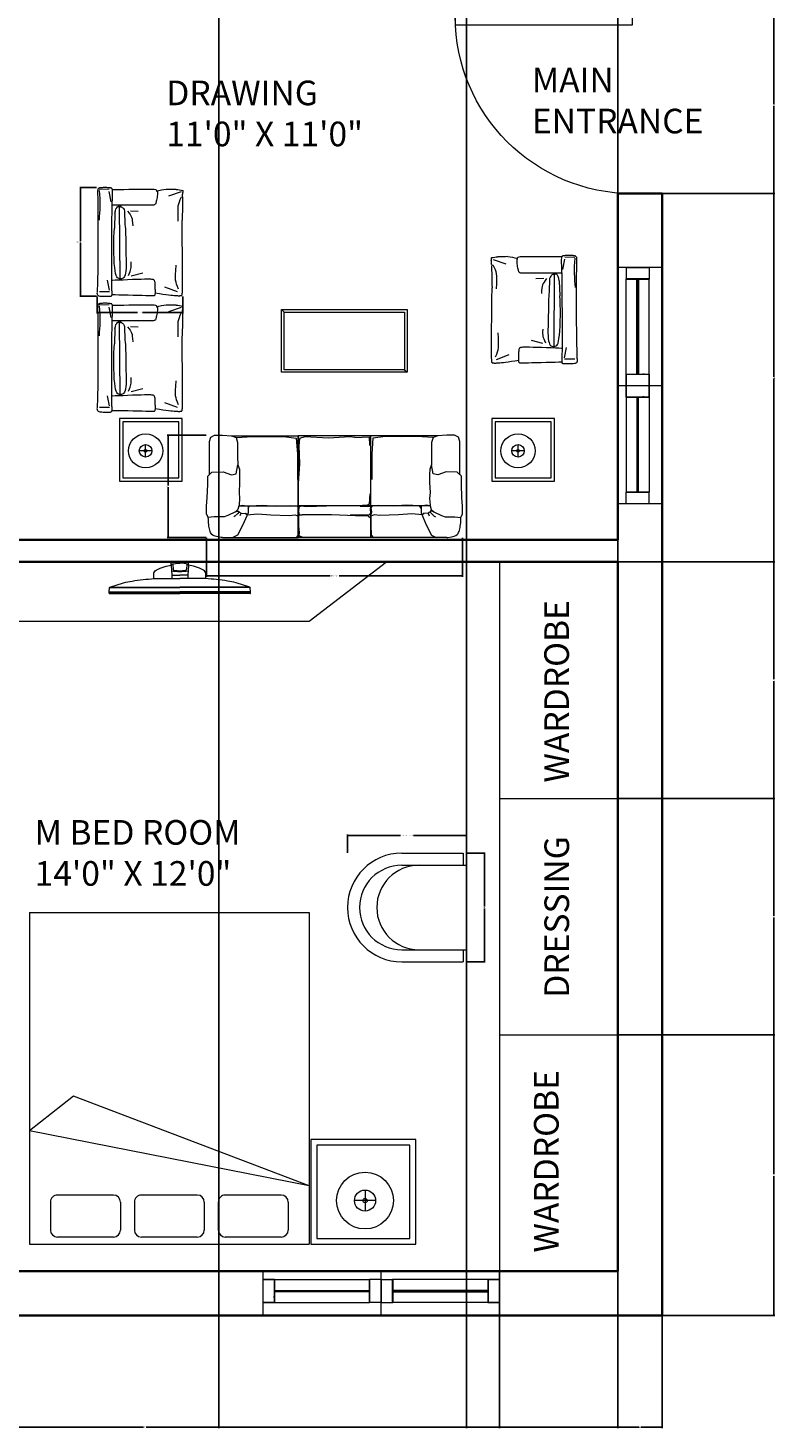
# Model space of a CAD drawing. Units: inches. Extents: x 1723 to 2209, y 1326 to 1810.
# Tile 5 of 6: x 2057 to 2209, y 1326 to 1610. Entities that reach past the tile are written whole.
import ezdxf

# ---------------------------------------------------------------- set-up
doc = ezdxf.new("R2010")
doc.units = ezdxf.units.IN
doc.layers.get('Defpoints').update_dxf_attribs({"color": 255})
for name, color, linetype, lineweight in [('A-ANNO-DIMS', 2, 'Continuous', 18), ('A-ANNO-TEXT', 7, 'Continuous', 18), ('A-AREA-IDEN', 7, 'Continuous', 18), ('A-DOOR', 3, 'Continuous', 18), ('A-EQPM', 8, 'Continuous', 13), ('A-FLOR-CASE', 9, 'Continuous', 18), ('A-FURN', 8, 'Continuous', 13), ('A-GLAZ', 4, 'Continuous', 18), ('A-WALL', 7, 'Continuous', 35), ('Sliding Door', 3, 'Continuous', 18)]:
    doc.layers.add(name, color=color, linetype=linetype, lineweight=lineweight)
doc.styles.get("Standard").update_dxf_attribs({"font": 'arial.ttf'})
doc.dimstyles.get("Standard").update_dxf_attribs({"dimtxt": 0.18, "dimasz": 0.18, "dimexe": 0.18, "dimexo": 0.0625, "dimgap": 0.09, "dimtad": 0, "dimtih": 1, "dimtoh": 1, "dimdec": 4, "dimzin": 0, "dimdsep": 46, "dimtxsty": 'Standard', "dimcen": 0.09, "dimadec": 0, "dimazin": 0, "dimtfac": 1, "dimtdec": 4, "dimtofl": 0, "dimtmove": 0, "dimatfit": 3, "dimfxl": 1, "dimtolj": 1, "dimtzin": 0, "dimarcsym": 0})

# ---------------------------------------------------------------- blocks, each defined once
blk = doc.blocks.new('armchair 042')
at = {"color": 0}
for p, q in [((672, 990), (673, 1002)), ((672, 985), (672, 990)), ((677, 823), (672, 985)), ((673, 1010), (674, 1014)), ((673, 1002), (673, 1010)), ((674, 1014), (675, 1017)), ((675, 1017), (676, 1020)), ((676, 1020), (678, 1023)), ((678, 1023), (680, 1025)), ((680, 1025), (684, 1026)), ((684, 1026), (688, 1027)), ((688, 1027), (694, 1029)), ((694, 1029), (700, 1029)), ((700, 1029), (709, 1030)), ((709, 1030), (718, 1030)), ((718, 1030), (728, 1031)), ((728, 1031), (739, 1031)), ((739, 1031), (750, 1031)), ((750, 1031), (760, 1031)), ((760, 1031), (770, 1030)), ((770, 1030), (779, 1030)), ((779, 1030), (787, 1029)), ((787, 1029), (793, 1028)), ((793, 1028), (798, 1027)), ((798, 1027), (803, 1025)), ((803, 1025), (806, 1023)), ((806, 1023), (809, 1020)), ((809, 1020), (811, 1016)), ((811, 1016), (813, 1011)), ((813, 1011), (814, 1005)), ((815, 997), (813, 908)), ((814, 1005), (815, 997)), ((557, 808), (554, 678)), ((562, 820), (557, 808)), ((568, 830), (562, 820)), ((574, 837), (568, 830)), ((580, 842), (574, 837)), ((587, 846), (580, 842)), ((595, 848), (587, 846)), ((599, 854), (591, 853)), ((602, 850), (595, 848)), ((607, 855), (599, 854)), ((610, 850), (602, 850)), ((614, 854), (607, 855)), ((618, 849), (610, 850)), ((622, 850), (614, 854)), ((625, 846), (618, 849)), ((629, 843), (622, 850)), ((632, 839), (625, 846)), ((639, 827), (632, 839)), ((645, 810), (639, 827)), ((650, 786), (645, 810)), ((678, 701), (677, 823)), ((812, 827), (811, 762)), ((813, 908), (812, 827)), ((7, 656), (8, 675)), ((8, 714), (8, 718)), ((8, 709), (8, 714)), ((8, 690), (8, 709)), ((8, 675), (8, 690)), ((554, 678), (551, 659)), ((650, 786), (654, 642)), ((679, 584), (678, 701)), ((811, 762), (811, 680)), ((811, 680), (811, 600)), ((7, 632), (7, 656)), ((7, 602), (7, 632)), ((7, 567), (7, 602)), ((7, 528), (7, 567)), ((547, 584), (546, 554)), ((546, 554), (546, 523)), ((548, 612), (547, 584)), ((549, 637), (548, 612)), ((551, 659), (549, 637)), ((657, 603), (654, 642)), ((659, 557), (657, 603)), ((660, 507), (659, 557)), ((680, 474), (679, 584)), ((811, 600), (812, 523)), ((4, 359), (5, 404)), ((5, 404), (7, 528)), ((545, 421), (544, 386)), ((546, 490), (545, 456)), ((545, 456), (545, 421)), ((546, 523), (546, 490)), ((657, 353), (659, 403)), ((659, 403), (660, 455)), ((660, 455), (660, 507)), ((680, 378), (680, 474)), ((812, 523), (812, 450)), ((812, 450), (812, 381)), ((4, 316), (4, 359)), ((4, 275), (4, 316)), ((4, 237), (4, 275)), ((543, 352), (542, 319)), ((542, 319), (542, 288)), ((542, 288), (543, 260)), ((544, 386), (543, 352)), ((651, 267), (655, 307)), ((655, 307), (657, 353)), ((680, 298), (680, 378)), ((680, 233), (680, 298)), ((812, 381), (813, 318)), ((813, 318), (813, 261)), ((4, 203), (4, 237)), ((4, 172), (4, 203)), ((4, 145), (4, 172)), ((4, 123), (4, 145)), ((543, 260), (545, 234)), ((545, 234), (548, 213)), ((548, 213), (552, 196)), ((552, 196), (558, 183)), ((558, 183), (564, 173)), ((564, 173), (572, 166)), ((572, 166), (579, 162)), ((579, 162), (588, 160)), ((588, 160), (596, 159)), ((596, 159), (604, 160)), ((604, 160), (611, 161)), ((611, 161), (619, 164)), ((619, 164), (625, 169)), ((625, 169), (632, 178)), ((632, 178), (638, 191)), ((638, 191), (643, 210)), ((643, 210), (647, 235)), ((647, 235), (651, 267)), ((680, 182), (680, 233)), ((680, 143), (680, 182)), ((680, 113), (680, 143)), ((813, 261), (814, 212)), ((814, 212), (815, 171)), ((815, 171), (816, 137)), ((816, 137), (816, 110)), ((4, 105), (4, 123)), ((4, 90), (4, 105)), ((4, 78), (4, 90)), ((4, 69), (4, 78)), ((4, 61), (4, 69)), ((4, 54), (4, 61)), ((4, 48), (4, 54)), ((4, 43), (4, 48)), ((5, 37), (4, 43)), ((5, 31), (5, 37)), ((5, 26), (5, 31)), ((6, 21), (5, 26)), ((6, 16), (6, 21)), ((7, 12), (6, 16)), ((7, 9), (7, 12)), ((8, 6), (7, 9)), ((9, 4), (8, 6)), ((9, 3), (9, 4)), ((10, 2), (9, 3)), ((11, 1), (10, 2)), ((12, 1), (11, 1)), ((13, 1), (12, 1)), ((14, 1), (13, 1)), ((15, 0), (14, 1)), ((16, 0), (15, 0)), ((18, 0), (16, 0)), ((70, 0), (59, -1)), ((82, 1), (70, 0)), ((98, 3), (82, 1)), ((116, 4), (98, 3)), ((137, 7), (116, 4)), ((163, 10), (137, 7)), ((192, 14), (163, 10)), ((225, 19), (192, 14)), ((264, 24), (225, 19)), ((677, 37), (678, 48)), ((677, 28), (677, 37)), ((677, 20), (677, 28)), ((677, 13), (677, 20)), ((677, 8), (677, 13)), ((678, 3), (677, 8)), ((678, 60), (679, 73)), ((678, 48), (678, 60)), ((679, -1), (678, 3)), ((679, 90), (680, 113)), ((679, 73), (679, 90)), ((797, 39), (701, 38)), ((814, 3), (809, 0)), ((817, 7), (814, 3)), ((816, 110), (817, 88)), ((817, 88), (818, 71)), ((819, 12), (817, 7)), ((818, 71), (819, 58)), ((819, 58), (819, 47)), ((819, 47), (820, 39)), ((820, 17), (819, 12)), ((820, 39), (820, 31)), ((820, 31), (821, 24)), ((821, 24), (820, 17)), ((19, 0), (18, 0)), ((21, -1), (19, 0)), ((23, -1), (21, -1)), ((25, -1), (23, -1)), ((27, -1), (25, -1)), ((29, -2), (27, -1)), ((31, -2), (29, -2)), ((35, -2), (31, -2)), ((39, -2), (35, -2)), ((44, -2), (39, -2)), ((51, -1), (44, -2)), ((59, -1), (51, -1)), ((681, -3), (679, -1)), ((684, -5), (681, -3)), ((687, -7), (684, -5)), ((691, -8), (687, -7)), ((696, -8), (691, -8)), ((702, -8), (696, -8)), ((709, -8), (702, -8)), ((718, -8), (709, -8)), ((728, -8), (718, -8)), ((739, -8), (728, -8)), ((750, -8), (739, -8)), ((762, -8), (750, -8)), ((773, -7), (762, -8)), ((784, -6), (773, -7)), ((794, -5), (784, -6)), ((802, -3), (794, -5)), ((809, 0), (802, -3))]:
    blk.add_line(p, q, dxfattribs=at)
for points in [[(16, 939), (28, 914), (37, 893), (43, 874), (47, 854), (49, 830), (50, 800), (49, 761), (47, 710)], [(17, 991), (139, 950)], [(674, 1014), (664, 1014), (641, 1014), (606, 1014), (564, 1014), (517, 1015), (468, 1015), (421, 1016), (378, 1016), (343, 1016), (314, 1016), (292, 1016), (275, 1015), (263, 1012), (254, 1008), (249, 1003), (245, 996), (244, 986), (243, 975), (244, 962), (245, 949), (247, 936), (249, 923), (252, 911), (254, 901), (256, 892), (258, 885), (259, 879), (261, 874), (264, 871), (267, 868), (270, 866), (274, 865), (280, 864), (291, 863), (310, 862), (343, 862), (391, 862), (460, 862), (553, 863), (673, 864)], [(685, 895), (703, 994)], [(703, 1015), (799, 1013)], [(799, 1004), (795, 964), (792, 926), (792, 890), (792, 855), (794, 820), (796, 787), (799, 754), (801, 721)], [(502, 809), (426, 805)], [(529, 807), (514, 788), (504, 773), (496, 760), (490, 747), (486, 733), (484, 715), (481, 693), (479, 664)], [(600, 160), (605, 850)], [(41, 60), (53, 85), (61, 107), (66, 126), (70, 146), (71, 170), (70, 200), (68, 239), (65, 290)], [(520, 191), (511, 212), (504, 229), (499, 243), (496, 256), (495, 268), (494, 283), (494, 301), (495, 323)], [(677, 8), (669, 8), (646, 8), (612, 7), (570, 6), (524, 5), (476, 4), (430, 3), (389, 2), (355, 1), (329, 0), (309, -1), (294, -1), (284, -1), (277, -1), (272, 0), (269, 2), (267, 4), (266, 7), (265, 11), (264, 16), (263, 22), (263, 28), (263, 35), (263, 43), (263, 52), (264, 61), (264, 71), (264, 81), (264, 90), (265, 100), (265, 108), (266, 116), (266, 123), (267, 129), (268, 134), (270, 139), (271, 142), (273, 145), (276, 148), (279, 150), (283, 152), (288, 153), (296, 154), (306, 155), (321, 156), (341, 156), (366, 155), (399, 154), (438, 153), (482, 152), (528, 150), (572, 148), (613, 146), (647, 145), (671, 144), (680, 144)], [(493, 189), (384, 216)], [(701, 50), (720, 148)], [(51, 36), (172, 81)]]:
    blk.add_lwpolyline(points, dxfattribs=at)
for centre, radius, start, end in [((57, 993), 57, 170.3495, 189.4629), ((4, 1002), 3.43, 101.0702, 170.3495), ((-256, 941), 260, 0.5509, 9.4629), ((159, 182), 837, 96.5918, 100.7196), ((4370, 902), 4366, 179.458, 182.4099), ((770, -30414), 31437, 91.1145, 91.2881), ((118, 571), 447, 72.4885, 84.8095)]:
    blk.add_arc(centre, radius, start, end, dxfattribs=at)
blk = doc.blocks.new('sofa 053')
at = {"color": 0}
for p, q in [((-920, 900), (188, 900)), ((-326, 0), (-326, 900)), ((-318, 814), (-313, 892)), ((-185, 886), (-313, 892)), ((-185, 886), (-140, 891)), ((-140, 891), (49, 880)), ((49, 880), (260, 891)), ((188, 900), (317, 900)), ((260, 891), (306, 877)), ((306, 877), (311, 812)), ((317, 0), (317, 900)), ((317, 900), (317, 0)), ((910, 900), (317, 900)), ((311, 812), (306, 652)), ((306, 652), (317, 477)), ((-851, 280), (188, 280)), ((188, 280), (317, 280)), ((842, 280), (317, 280)), ((143, 201), (209, 202)), ((209, 202), (282, 201)), ((-998, 0), (188, 0)), ((188, 0), (317, 0)), ((989, 0), (317, 0))]:
    blk.add_line(p, q, dxfattribs=at)
for points in [[(-1112, 556), (-1113, 849), (-1101, 889), (-1067, 906), (-997, 906), (-918, 900), (-876, 886), (-864, 841), (-864, 717), (-862, 643)], [(-876, 886), (-729, 894)], [(-598, 891), (-455, 894), (-344, 880), (-333, 742), (-333, 513)], [(720, 894), (445, 894), (335, 880), (324, 742), (324, 513)], [(866, 886), (720, 894)], [(1103, 556), (1103, 849), (1092, 889), (1058, 906), (988, 906), (909, 900), (866, 886), (855, 841), (855, 717), (853, 643)], [(-983, 183), (-1070, 183), (-1123, 178), (-1138, 209), (-1138, 277), (-1132, 353), (-1127, 468), (-1127, 542), (-1090, 578), (-991, 581), (-918, 556), (-876, 564), (-862, 643), (-862, 643), (-847, 601)], [(-862, 643), (-847, 606), (-845, 554), (-845, 488), (-850, 397), (-845, 345), (-850, 286), (-851, 280)], [(853, 643), (838, 606), (836, 554), (836, 488), (840, 397), (836, 345), (840, 286), (842, 280)], [(974, 183), (1061, 183), (1114, 178), (1129, 209), (1129, 277), (1123, 353), (1118, 468), (1118, 542), (1081, 578), (982, 581), (909, 556), (866, 564), (853, 643), (853, 643), (838, 601)], [(-318, 388), (-312, 296), (-300, 287), (-202, 280)], [(-851, 280), (-861, 248), (-882, 227), (-951, 195), (-983, 183)], [(-851, 280), (-819, 285), (-771, 277), (-771, 217), (-816, 113), (-864, 20), (-904, 0)], [(-771, 259), (-757, 279), (-639, 285), (-522, 278), (-394, 284), (-337, 281), (-326, 262), (-331, 225), (-326, 200)], [(-142, 202), (-318, 205), (-326, 215), (-322, 250), (-325, 271), (-230, 275)], [(67, 277), (241, 272), (295, 278), (313, 269), (316, 229), (310, 202), (282, 201), (314, 195), (317, 133), (310, 42), (312, 18), (286, 5)], [(762, 259), (748, 279), (630, 285), (513, 278), (385, 284), (327, 281), (317, 262), (321, 225), (317, 200)], [(842, 280), (810, 285), (762, 277), (762, 217), (807, 113), (855, 20), (895, 0)], [(842, 280), (852, 248), (873, 227), (942, 195), (974, 183)], [(-998, 0), (-1008, 1), (-1039, 6), (-1062, 12), (-1079, 19), (-1091, 26), (-1098, 35), (-1103, 44), (-1107, 54), (-1110, 65), (-1113, 76), (-1115, 88), (-1117, 101), (-1119, 115), (-1121, 129), (-1122, 144), (-1123, 161), (-1123, 178)], [(-882, 227), (-866, 232), (-851, 232), (-851, 223), (-862, 212), (-887, 190), (-897, 182)], [(-851, 223), (-838, 222), (-833, 211), (-843, 192)], [(-833, 211), (-794, 214), (-788, 207), (-779, 200)], [(-779, 200), (-687, 209), (-570, 200), (-406, 194), (-354, 201), (-325, 189), (-324, 108), (-329, 21), (-346, 0)], [(-324, 168), (-301, 190), (-191, 193), (24, 201), (143, 201)], [(769, 200), (677, 209), (561, 200), (397, 194), (345, 201), (316, 189), (314, 108), (319, 21), (337, 0)], [(824, 211), (784, 214), (779, 207), (769, 200)], [(842, 223), (829, 222), (824, 211), (833, 192)], [(873, 227), (857, 232), (842, 232), (842, 223), (853, 212), (878, 190), (888, 182)], [(989, 0), (999, 1), (1030, 6), (1053, 12), (1070, 19), (1082, 26), (1089, 35), (1094, 44), (1098, 54), (1101, 65), (1104, 76), (1106, 88), (1108, 101), (1110, 115), (1112, 129), (1113, 144), (1113, 161), (1114, 178)]]:
    blk.add_lwpolyline(points, dxfattribs=at)
at = {"color": 0, "flags": 128}
blk.add_lwpolyline([(-729, 894), (-598, 891)], dxfattribs=at)
blk = doc.blocks.new('A$C793B20D3')
for p, q in [((0.625, -0.395), (0.625, 1.975)), ((2.625, 1.975), (0.625, 1.975)), ((0.825, 1.925), (1.225, 1.925)), ((1.425, 1.925), (1.825, 1.925)), ((2.025, 1.925), (2.425, 1.925)), ((2.625, -0.395), (2.625, 1.975)), ((0.775, 1.675), (0.775, 1.875)), ((1.275, 1.675), (1.275, 1.875)), ((1.375, 1.675), (1.375, 1.875)), ((1.875, 1.675), (1.875, 1.875)), ((1.975, 1.675), (1.975, 1.875)), ((2.475, 1.675), (2.475, 1.875)), ((0.825, 1.625), (1.225, 1.625)), ((1.425, 1.625), (1.825, 1.625)), ((2.025, 1.625), (2.425, 1.625)), ((0.626, 1.56), (2.311, 0.917)), ((0.626, 1.56), (2.625, 1.165)), ((2.311, 0.917), (2.625, 1.165)), ((2.625, -0.395), (0.625, -0.395))]:
    blk.add_line(p, q)
for centre, start, end in [((0.825, 1.875), 90, 180), ((1.225, 1.875), 0, 90), ((1.425, 1.875), 90, 180), ((1.825, 1.875), 0, 90), ((2.025, 1.875), 90, 180), ((2.425, 1.875), 0, 90), ((0.825, 1.675), 180, 270), ((1.225, 1.675), 270, 0), ((1.425, 1.675), 180, 270), ((1.825, 1.675), 270, 0), ((2.025, 1.675), 180, 270), ((2.425, 1.675), 270, 0)]:
    blk.add_arc(centre, 0.05, start, end)
blk = doc.blocks.new('B1')
at = {"color": 0}
for points in [[(-24.5, 37.9), (-24.5, 43.2, -0.236854), (-23.9, 44.5, -0.069077), (0, 47.8, -0.069077)], [(-24.5, 37.7), (-24.5, 38.9, -0.236854), (-23.9, 40.2, -0.069077), (0, 43.6, -0.069077)], [(24.5, 37.9), (24.5, 43.2, 0.236854), (23.9, 44.5, 0.069077), (0, 47.8, 0.069077)], [(24.5, 37.7), (24.5, 38.9, 0.236854), (23.9, 40.2, 0.069077), (0, 43.6, 0.069077)], [(-200, -38.4), (-200, -37.7), (-199.2, -25.8, -0.303983), (-198.5, -24.8), (-159.1, -12.4, -0.039649), (-135.4, -7, -0.017831), (-72.5, 0), (0, 0)], [(-73.6, -0.1), (-73.6, 13.1, -0.272026), (-67.3, 23.9, -0.059641), (-43.9, 33.5, -0.024069), (-24.5, 37.9), (-22.7, 10), (-22.7, 0)], [(200, -38.4), (200, -37.7), (199.2, -25.8, 0.303983), (198.5, -24.8), (159.1, -12.4, 0.039649), (135.4, -7, 0.017831), (72.5, 0), (0, 0)], [(73.6, -0.1), (73.6, 13.1, 0.272026), (67.3, 23.9, 0.059641), (43.9, 33.5, 0.024069), (24.5, 37.9), (22.7, 10), (22.7, 0)]]:
    blk.add_lwpolyline(points, format="xyb", dxfattribs=at)
for points in [[(-19.8, 40.1), (-18.9, 26.4)], [(19.8, 40.1), (18.9, 26.4)], [(-22.7, 10), (0, 10)], [(22.7, 10), (0, 10)], [(-200, -37.8), (0, -37.8)], [(-200, -41.4), (-200, -38.4), (200, -38.4)], [(-200, -38.4), (0, -38.4)], [(200, -41.4), (200, -38.4), (-200, -38.4)], [(-199.2, -25.8), (0, -25.8)], [(-196.3, -24.2), (0, -24.2)], [(196.3, -24.2), (0, -24.2)], [(199.2, -25.8), (0, -25.8)], [(200, -37.8), (0, -37.8)], [(200, -38.4), (0, -38.4)], [(-198.9, -42.4), (0, -42.4)], [(198.9, -42.4), (0, -42.4)]]:
    blk.add_lwpolyline(points, dxfattribs=at)
for centre, radius, start, end in [((0, 150), 130, 259.5789, 270), ((-15.4, 26.6), 3.53, 183.678, 262.9963), ((0, 152.2), 130, 262.9963, 270), ((0, 152.2), 130, 270, 277.0037), ((0, 150), 130, 270, 280.4211), ((15.4, 26.6), 3.53, 277.0037, 356.322), ((-198.9, -41.4), 1.06, 180, 270), ((198.9, -41.4), 1.06, 270, 0)]:
    blk.add_arc(centre, radius, start, end, dxfattribs=at)
blk = doc.blocks.new('armchair032')
at = {"color": 0}
for p, q in [((-315, 375), (-315, 20)), ((-245, 375), (-245, 0)), ((245, 375), (245, 0)), ((315, 375), (315, 20)), ((-245, 20), (-315, 20)), ((245, 0), (-245, 0)), ((315, 20), (245, 20))]:
    blk.add_line(p, q, dxfattribs=at)
for centre, radius in [((0, 375), 315), ((0, 375), 245), ((0, 275), 245)]:
    blk.add_arc(centre, radius, 0.00003, 179.99998, dxfattribs=at)
blk = doc.blocks.new('*U41')
for p, q in [((0, 0), (0, -6)), ((36, 0), (36, -6))]:
    blk.add_line(p, q)
blk.add_lwpolyline([(0, 0), (0, 36), (1.75, 36), (1.75, 0)], close=True)
blk.add_arc((0, 0), 36, 0, 90)
blk = doc.blocks.new('SW')
blk.add_line((2331.37, 1559.31), (2331.37, 1550.31))
at = {"layer": 'Sliding Door'}
for p, q in [((2285.07, 1559.31), (2285.07, 1550.31)), ((2285.07, 1559.31), (2285.07, 1550.31)), ((2285.07, 1559.31), (2289.58, 1559.31)), ((2289.51, 1550.31), (2289.51, 1559.31)), ((2331.37, 1559.31), (2289.51, 1559.31)), ((2289.58, 1559.31), (2289.58, 1550.31)), ((2326.86, 1555.09), (2289.58, 1555.09)), ((2289.58, 1554.81), (2326.86, 1554.81)), ((2326.86, 1559.31), (2326.86, 1550.31)), ((2326.86, 1559.31), (2331.37, 1559.31)), ((2326.93, 1559.31), (2326.93, 1550.31)), ((2285.07, 1550.31), (2289.51, 1550.31)), ((2285.07, 1550.31), (2289.58, 1550.31)), ((2331.37, 1550.31), (2289.51, 1550.31)), ((2289.58, 1554.53), (2326.86, 1554.53)), ((2289.58, 1552.81), (2289.58, 1552.25)), ((2326.86, 1550.31), (2331.37, 1550.31)), ((2326.93, 1552.25), (2326.93, 1552.81)), ((2326.93, 1550.31), (2331.37, 1550.31))]:
    blk.add_line(p, q, dxfattribs=at)
blk = doc.blocks.new('TABLE-END-SMALL')
for p, q in [((6.6, 6.17), (4.03, 6.17)), ((5.32, 4.88), (5.32, 7.45))]:
    blk.add_line(p, q)
for points in [[(0, 0), (12.75, 0), (12.75, 12.75), (0, 12.75)], [(0.71, 0.71), (12.04, 0.71), (12.04, 12.04), (0.71, 12.04)]]:
    blk.add_lwpolyline(points, close=True)
for radius in [3.46, 1.28, 0.266]:
    blk.add_circle((5.32, 6.17), radius)
blk = doc.blocks.new('TABLE-END-LARGE')
for p, q in [((12.41, 13.14), (12.41, 8.85)), ((10.27, 10.99), (14.56, 10.99))]:
    blk.add_line(p, q)
for points in [[(21.29, 21.29), (0, 21.29), (0, 0), (21.29, 0)], [(20.1, 20.1), (1.18, 20.1), (1.18, 1.18), (20.1, 1.18)]]:
    blk.add_lwpolyline(points, close=True)
for radius in [5.77, 2.14, 0.445]:
    blk.add_circle((12.41, 10.99), radius)
blk = doc.blocks.new('TABLE-COFFEE-RECT')
for p, q in [((0, 0), (0, 12.75)), ((0, 12.75), (0.53, 12.22)), ((0, 12.75), (25.5, 12.75)), ((0.53, 0.53), (0.53, 12.22)), ((0.53, 12.22), (24.97, 12.22)), ((24.97, 12.22), (24.97, 0.53)), ((25.5, 12.75), (25.5, 0)), ((25.5, 0), (0, 0)), ((24.97, 0.53), (0.53, 0.53)), ((24.97, 0.53), (25.5, 0))]:
    blk.add_line(p, q)
blk = doc.blocks.new('*D59')
at = {"layer": 'A-ANNO-DIMS', "color": 0, "lineweight": -2, "transparency": 16777216}
for p, q in [((2070.83, 1577.71), (2067.4, 1577.71)), ((2067.58, 1577.53), (2067.58, 1566.85)), ((2067.58, 1555.81), (2067.58, 1566.48)), ((2070.83, 1555.63), (2067.4, 1555.63))]:
    blk.add_line(p, q, dxfattribs=at)
at = {"layer": 'A-ANNO-DIMS', "color": 0, "transparency": 16777216}
for points in [[(2067.55, 1577.53), (2067.61, 1577.53), (2067.58, 1577.71)], [(2067.55, 1555.81), (2067.61, 1555.81), (2067.58, 1555.63)]]:
    blk.add_solid(points, dxfattribs=at)
at = {"layer": 'Defpoints', "color": 0, "transparency": 16777216}
for p in [(2067.58, 1577.71), (2070.9, 1577.71), (2070.9, 1555.63)]:
    blk.add_point(p, dxfattribs=at)
at = {"layer": 'A-ANNO-DIMS', "color": 0, "transparency": 16777216, "insert": (2067.58, 1566.67), "char_height": 0.18, "attachment_point": 5}
blk.add_mtext('\\A1;ARMCHAIR 22 TYP.', dxfattribs=at)
blk = doc.blocks.new('*D60')
at = {"layer": 'A-ANNO-DIMS', "color": 0, "lineweight": -2, "transparency": 16777216}
for p, q in [((2070.9, 1555.56), (2070.9, 1552.14)), ((2088.34, 1555.56), (2088.34, 1552.14)), ((2071.08, 1552.32), (2079.1, 1552.32)), ((2088.16, 1552.32), (2080.14, 1552.32))]:
    blk.add_line(p, q, dxfattribs=at)
at = {"layer": 'A-ANNO-DIMS', "color": 0, "transparency": 16777216}
for points in [[(2071.08, 1552.35), (2071.08, 1552.29), (2070.9, 1552.32)], [(2088.16, 1552.35), (2088.16, 1552.29), (2088.34, 1552.32)]]:
    blk.add_solid(points, dxfattribs=at)
at = {"layer": 'Defpoints', "color": 0, "transparency": 16777216}
for p in [(2070.9, 1555.63), (2088.34, 1555.63), (2070.9, 1552.32)]:
    blk.add_point(p, dxfattribs=at)
at = {"layer": 'A-ANNO-DIMS', "color": 0, "transparency": 16777216, "insert": (2079.62, 1552.32), "char_height": 0.18, "attachment_point": 5}
blk.add_mtext('\\A1;17 TYP.', dxfattribs=at)
blk = doc.blocks.new('*D73')
at = {"layer": 'A-ANNO-DIMS', "color": 0, "lineweight": -2, "transparency": 16777216}
for p, q in [((2093.14, 1506.6), (2093.14, 1498.69)), ((2145.11, 1506.6), (2145.11, 1498.69)), ((2093.32, 1498.87), (2118.22, 1498.87)), ((2144.93, 1498.87), (2120.03, 1498.87))]:
    blk.add_line(p, q, dxfattribs=at)
at = {"layer": 'A-ANNO-DIMS', "color": 0, "transparency": 16777216}
for points in [[(2093.32, 1498.9), (2093.32, 1498.84), (2093.14, 1498.87)], [(2144.93, 1498.9), (2144.93, 1498.84), (2145.11, 1498.87)]]:
    blk.add_solid(points, dxfattribs=at)
at = {"layer": 'Defpoints', "color": 0, "transparency": 16777216}
for p in [(2093.14, 1506.66), (2145.11, 1506.66), (2093.14, 1498.87)]:
    blk.add_point(p, dxfattribs=at)
at = {"layer": 'A-ANNO-DIMS', "color": 0, "transparency": 16777216, "insert": (2119.12, 1498.87), "char_height": 0.18, "attachment_point": 5}
blk.add_mtext('\\A1;SOFA 52 TYP.', dxfattribs=at)
blk = doc.blocks.new('*D74')
at = {"layer": 'A-ANNO-DIMS', "color": 0, "lineweight": -2, "transparency": 16777216}
for p, q in [((2093.07, 1527.42), (2085.16, 1527.42)), ((2085.34, 1527.24), (2085.34, 1517.22)), ((2085.34, 1506.84), (2085.34, 1516.86)), ((2093.07, 1506.66), (2085.16, 1506.66))]:
    blk.add_line(p, q, dxfattribs=at)
at = {"layer": 'A-ANNO-DIMS', "color": 0, "transparency": 16777216}
for points in [[(2085.31, 1527.24), (2085.37, 1527.24), (2085.34, 1527.42)], [(2085.31, 1506.84), (2085.37, 1506.84), (2085.34, 1506.66)]]:
    blk.add_solid(points, dxfattribs=at)
at = {"layer": 'Defpoints', "color": 0, "transparency": 16777216}
for p in [(2085.34, 1527.42), (2093.14, 1527.42), (2093.14, 1506.66)]:
    blk.add_point(p, dxfattribs=at)
at = {"layer": 'A-ANNO-DIMS', "color": 0, "transparency": 16777216, "insert": (2085.34, 1517.04), "char_height": 0.18, "attachment_point": 5}
blk.add_mtext('\\A1;21 TYP.', dxfattribs=at)
blk = doc.blocks.new('*D89')
at = {"layer": 'A-ANNO-DIMS', "color": 0, "lineweight": -2, "transparency": 16777216}
for p, q in [((2121.74, 1442.62), (2121.74, 1446.36)), ((2121.92, 1446.18), (2132.49, 1446.18)), ((2145.72, 1446.18), (2135.15, 1446.18)), ((2145.9, 1442.62), (2145.9, 1446.36))]:
    blk.add_line(p, q, dxfattribs=at)
at = {"layer": 'A-ANNO-DIMS', "color": 0, "transparency": 16777216}
for points in [[(2121.92, 1446.21), (2121.92, 1446.15), (2121.74, 1446.18)], [(2145.72, 1446.21), (2145.72, 1446.15), (2145.9, 1446.18)]]:
    blk.add_solid(points, dxfattribs=at)
at = {"layer": 'Defpoints', "color": 0, "transparency": 16777216}
for p in [(2121.74, 1446.18), (2121.74, 1442.56), (2145.9, 1442.56)]:
    blk.add_point(p, dxfattribs=at)
at = {"layer": 'A-ANNO-DIMS', "color": 0, "transparency": 16777216, "insert": (2133.82, 1446.18), "char_height": 0.18, "attachment_point": 5}
blk.add_mtext('\\A1;DRESSING CHAIR 24', dxfattribs=at)
blk = doc.blocks.new('*D90')
at = {"layer": 'A-ANNO-DIMS', "color": 0, "lineweight": -2, "transparency": 16777216}
for p, q in [((2145.96, 1442.56), (2149.7, 1442.56)), ((2149.52, 1442.38), (2149.52, 1431.71)), ((2149.52, 1420.68), (2149.52, 1431.35)), ((2145.96, 1420.5), (2149.7, 1420.5))]:
    blk.add_line(p, q, dxfattribs=at)
at = {"layer": 'A-ANNO-DIMS', "color": 0, "transparency": 16777216}
for points in [[(2149.49, 1442.38), (2149.55, 1442.38), (2149.52, 1442.56)], [(2149.49, 1420.68), (2149.55, 1420.68), (2149.52, 1420.5)]]:
    blk.add_solid(points, dxfattribs=at)
at = {"layer": 'Defpoints', "color": 0, "transparency": 16777216}
for p in [(2145.9, 1442.56), (2149.52, 1442.56), (2145.9, 1420.5)]:
    blk.add_point(p, dxfattribs=at)
at = {"layer": 'A-ANNO-DIMS', "color": 0, "transparency": 16777216, "insert": (2149.52, 1431.53), "char_height": 0.18, "attachment_point": 5}
blk.add_mtext('\\A1;22', dxfattribs=at)
blk = doc.blocks.new('*D98')
at = {"layer": 'A-ANNO-DIMS', "color": 0, "lineweight": -2, "transparency": 16777216}
for p, q in [((2152.6, 1357.63), (2152.6, 1325.84)), ((2008.6, 1348.63), (2008.6, 1325.84)), ((2008.78, 1326.02), (2080.32, 1326.02)), ((2152.42, 1326.02), (2080.88, 1326.02))]:
    blk.add_line(p, q, dxfattribs=at)
at = {"layer": 'A-ANNO-DIMS', "color": 0, "transparency": 16777216}
for points in [[(2008.78, 1326.05), (2008.78, 1325.99), (2008.6, 1326.02)], [(2152.42, 1326.05), (2152.42, 1325.99), (2152.6, 1326.02)]]:
    blk.add_solid(points, dxfattribs=at)
at = {"layer": 'Defpoints', "color": 0, "transparency": 16777216}
for p in [(2152.6, 1357.69), (2008.6, 1348.69), (2152.6, 1326.02)]:
    blk.add_point(p, dxfattribs=at)
at = {"layer": 'A-ANNO-DIMS', "color": 0, "transparency": 16777216, "insert": (2080.6, 1326.02), "char_height": 0.18, "attachment_point": 5}
blk.add_mtext('\\A1;144', dxfattribs=at)
blk = doc.blocks.new('*D99')
at = {"layer": 'A-ANNO-DIMS', "color": 0, "lineweight": -2, "transparency": 16777216}
for p, q in [((2152.6, 1357.63), (2152.6, 1325.84)), ((2176.6, 1357.63), (2176.6, 1325.84)), ((2152.78, 1326.02), (2164.38, 1326.02)), ((2176.42, 1326.02), (2164.82, 1326.02))]:
    blk.add_line(p, q, dxfattribs=at)
at = {"layer": 'A-ANNO-DIMS', "color": 0, "transparency": 16777216}
for points in [[(2152.78, 1326.05), (2152.78, 1325.99), (2152.6, 1326.02)], [(2176.42, 1326.05), (2176.42, 1325.99), (2176.6, 1326.02)]]:
    blk.add_solid(points, dxfattribs=at)
at = {"layer": 'Defpoints', "color": 0, "transparency": 16777216}
for p in [(2152.6, 1357.69), (2176.6, 1357.69), (2176.6, 1326.02)]:
    blk.add_point(p, dxfattribs=at)
at = {"layer": 'A-ANNO-DIMS', "color": 0, "transparency": 16777216, "insert": (2164.6, 1326.02), "char_height": 0.18, "attachment_point": 5}
blk.add_mtext('\\A1;24', dxfattribs=at)
blk = doc.blocks.new('*D100')
at = {"layer": 'A-ANNO-DIMS', "color": 0, "lineweight": -2, "transparency": 16777216}
for p, q in [((2176.6, 1357.63), (2176.6, 1325.84)), ((2185.6, 1348.63), (2185.6, 1325.84)), ((2176.78, 1326.02), (2180.95, 1326.02)), ((2185.42, 1326.02), (2181.25, 1326.02))]:
    blk.add_line(p, q, dxfattribs=at)
at = {"layer": 'A-ANNO-DIMS', "color": 0, "transparency": 16777216}
for points in [[(2176.78, 1326.05), (2176.78, 1325.99), (2176.6, 1326.02)], [(2185.42, 1326.05), (2185.42, 1325.99), (2185.6, 1326.02)]]:
    blk.add_solid(points, dxfattribs=at)
at = {"layer": 'Defpoints', "color": 0, "transparency": 16777216}
for p in [(2176.6, 1357.69), (2185.6, 1348.69), (2185.6, 1326.02)]:
    blk.add_point(p, dxfattribs=at)
at = {"layer": 'A-ANNO-DIMS', "color": 0, "transparency": 16777216, "insert": (2181.1, 1326.02), "char_height": 0.18, "attachment_point": 5}
blk.add_mtext('\\A1;9', dxfattribs=at)
blk = doc.blocks.new('*D102')
at = {"layer": 'A-ANNO-DIMS', "color": 0, "lineweight": -2, "transparency": 16777216}
for p, q in [((2185.67, 1612.49), (2208.45, 1612.49)), ((2208.27, 1612.31), (2208.27, 1594.67)), ((2208.27, 1576.67), (2208.27, 1594.3)), ((2185.67, 1576.49), (2208.45, 1576.49))]:
    blk.add_line(p, q, dxfattribs=at)
at = {"layer": 'A-ANNO-DIMS', "color": 0, "transparency": 16777216}
for points in [[(2208.24, 1612.31), (2208.3, 1612.31), (2208.27, 1612.49)], [(2208.24, 1576.67), (2208.3, 1576.67), (2208.27, 1576.49)]]:
    blk.add_solid(points, dxfattribs=at)
at = {"layer": 'Defpoints', "color": 0, "transparency": 16777216}
for p in [(2185.6, 1612.49), (2208.27, 1612.49), (2185.6, 1576.49)]:
    blk.add_point(p, dxfattribs=at)
at = {"layer": 'A-ANNO-DIMS', "color": 0, "transparency": 16777216, "insert": (2208.27, 1594.49), "char_height": 0.18, "attachment_point": 5}
blk.add_mtext('\\A1;36', dxfattribs=at)
blk = doc.blocks.new('*D103')
at = {"layer": 'A-ANNO-DIMS', "color": 0, "lineweight": -2, "transparency": 16777216}
for p, q in [((2185.67, 1576.49), (2208.45, 1576.49)), ((2208.27, 1576.31), (2208.27, 1539.27)), ((2208.27, 1501.87), (2208.27, 1538.91)), ((2176.67, 1501.69), (2208.45, 1501.69))]:
    blk.add_line(p, q, dxfattribs=at)
at = {"layer": 'A-ANNO-DIMS', "color": 0, "transparency": 16777216}
for points in [[(2208.24, 1576.31), (2208.3, 1576.31), (2208.27, 1576.49)], [(2208.24, 1501.87), (2208.3, 1501.87), (2208.27, 1501.69)]]:
    blk.add_solid(points, dxfattribs=at)
at = {"layer": 'Defpoints', "color": 0, "transparency": 16777216}
for p in [(2185.6, 1576.49), (2208.27, 1576.49), (2176.6, 1501.69)]:
    blk.add_point(p, dxfattribs=at)
at = {"layer": 'A-ANNO-DIMS', "color": 0, "transparency": 16777216, "insert": (2208.27, 1539.09), "char_height": 0.18, "attachment_point": 5}
blk.add_mtext('\\A1;74.8', dxfattribs=at)
blk = doc.blocks.new('*D104')
at = {"layer": 'A-ANNO-DIMS', "color": 0, "lineweight": -2, "transparency": 16777216}
for p, q in [((2176.67, 1501.69), (2208.45, 1501.69)), ((2208.27, 1501.51), (2208.27, 1477.87)), ((2208.27, 1453.87), (2208.27, 1477.51)), ((2176.67, 1453.69), (2208.45, 1453.69))]:
    blk.add_line(p, q, dxfattribs=at)
at = {"layer": 'A-ANNO-DIMS', "color": 0, "transparency": 16777216}
for points in [[(2208.24, 1501.51), (2208.3, 1501.51), (2208.27, 1501.69)], [(2208.24, 1453.87), (2208.3, 1453.87), (2208.27, 1453.69)]]:
    blk.add_solid(points, dxfattribs=at)
at = {"layer": 'Defpoints', "color": 0, "transparency": 16777216}
for p in [(2176.6, 1501.69), (2208.27, 1501.69), (2176.6, 1453.69)]:
    blk.add_point(p, dxfattribs=at)
at = {"layer": 'A-ANNO-DIMS', "color": 0, "transparency": 16777216, "insert": (2208.27, 1477.69), "char_height": 0.18, "attachment_point": 5}
blk.add_mtext('\\A1;48', dxfattribs=at)
blk = doc.blocks.new('*D105')
at = {"layer": 'A-ANNO-DIMS', "color": 0, "lineweight": -2, "transparency": 16777216}
for p, q in [((2176.67, 1453.69), (2208.45, 1453.69)), ((2208.27, 1453.51), (2208.27, 1429.87)), ((2208.27, 1405.87), (2208.27, 1429.51)), ((2176.67, 1405.69), (2208.45, 1405.69))]:
    blk.add_line(p, q, dxfattribs=at)
at = {"layer": 'A-ANNO-DIMS', "color": 0, "transparency": 16777216}
for points in [[(2208.24, 1453.51), (2208.3, 1453.51), (2208.27, 1453.69)], [(2208.24, 1405.87), (2208.3, 1405.87), (2208.27, 1405.69)]]:
    blk.add_solid(points, dxfattribs=at)
at = {"layer": 'Defpoints', "color": 0, "transparency": 16777216}
for p in [(2176.6, 1453.69), (2208.27, 1453.69), (2176.6, 1405.69)]:
    blk.add_point(p, dxfattribs=at)
at = {"layer": 'A-ANNO-DIMS', "color": 0, "transparency": 16777216, "insert": (2208.27, 1429.69), "char_height": 0.18, "attachment_point": 5}
blk.add_mtext('\\A1;48', dxfattribs=at)
blk = doc.blocks.new('*D106')
at = {"layer": 'A-ANNO-DIMS', "color": 0, "lineweight": -2, "transparency": 16777216}
for p, q in [((2176.67, 1405.69), (2208.45, 1405.69)), ((2208.27, 1405.51), (2208.27, 1377.37)), ((2208.27, 1348.87), (2208.27, 1377.01)), ((2185.67, 1348.69), (2208.45, 1348.69))]:
    blk.add_line(p, q, dxfattribs=at)
at = {"layer": 'A-ANNO-DIMS', "color": 0, "transparency": 16777216}
for points in [[(2208.24, 1405.51), (2208.3, 1405.51), (2208.27, 1405.69)], [(2208.24, 1348.87), (2208.3, 1348.87), (2208.27, 1348.69)]]:
    blk.add_solid(points, dxfattribs=at)
at = {"layer": 'Defpoints', "color": 0, "transparency": 16777216}
for p in [(2176.6, 1405.69), (2208.27, 1405.69), (2185.6, 1348.69)]:
    blk.add_point(p, dxfattribs=at)
at = {"layer": 'A-ANNO-DIMS', "color": 0, "transparency": 16777216, "insert": (2208.27, 1377.19), "char_height": 0.18, "attachment_point": 5}
blk.add_mtext('\\A1;57', dxfattribs=at)
blk = doc.blocks.new('*D113')
at = {"layer": 'A-ANNO-DIMS', "color": 0, "lineweight": -2, "transparency": 16777216}
for p, q in [((2095.65, 1657.63), (2095.65, 1325.84)), ((2176.6, 1657.63), (2176.6, 1325.84)), ((2095.83, 1326.02), (2135.73, 1326.02)), ((2176.42, 1326.02), (2136.52, 1326.02))]:
    blk.add_line(p, q, dxfattribs=at)
at = {"layer": 'A-ANNO-DIMS', "color": 0, "transparency": 16777216}
for points in [[(2095.83, 1326.05), (2095.83, 1325.99), (2095.65, 1326.02)], [(2176.42, 1326.05), (2176.42, 1325.99), (2176.6, 1326.02)]]:
    blk.add_solid(points, dxfattribs=at)
at = {"layer": 'Defpoints', "color": 0, "transparency": 16777216}
for p in [(2095.65, 1657.69), (2176.6, 1657.69), (2176.6, 1326.02)]:
    blk.add_point(p, dxfattribs=at)
at = {"layer": 'A-ANNO-DIMS', "color": 0, "transparency": 16777216, "insert": (2136.13, 1326.02), "char_height": 0.18, "attachment_point": 5}
blk.add_mtext('\\A1;80.95', dxfattribs=at)
blk = doc.blocks.new('*D115')
at = {"layer": 'A-ANNO-DIMS', "color": 0, "lineweight": -2, "transparency": 16777216}
for p, q in [((2145.93, 1777.63), (2145.93, 1325.84)), ((2176.6, 1777.63), (2176.6, 1325.84)), ((2146.11, 1326.02), (2160.8, 1326.02)), ((2176.42, 1326.02), (2161.73, 1326.02))]:
    blk.add_line(p, q, dxfattribs=at)
at = {"layer": 'A-ANNO-DIMS', "color": 0, "transparency": 16777216}
for points in [[(2146.11, 1326.05), (2146.11, 1325.99), (2145.93, 1326.02)], [(2176.42, 1326.05), (2176.42, 1325.99), (2176.6, 1326.02)]]:
    blk.add_solid(points, dxfattribs=at)
at = {"layer": 'Defpoints', "color": 0, "transparency": 16777216}
for p in [(2145.93, 1777.69), (2176.6, 1777.69), (2176.6, 1326.02)]:
    blk.add_point(p, dxfattribs=at)
at = {"layer": 'A-ANNO-DIMS', "color": 0, "transparency": 16777216, "insert": (2161.26, 1326.02), "char_height": 0.18, "attachment_point": 5}
blk.add_mtext('\\A1;30.677', dxfattribs=at)

msp = doc.modelspace()

# ---------------------------------------------------------------- linework, layer by layer
at = {"layer": 'A-FLOR-CASE'}
for p, q in [((2041.8437, 1501.6915), (2151.6826, 1501.6915)), ((2113.9849, 1489.6915), (2129.6458, 1501.6915)), ((2152.6032, 1501.6915), (2152.6032, 1357.6915)), ((2041.8437, 1489.6915), (2113.9849, 1489.6915)), ((2152.6032, 1453.6915), (2176.6032, 1453.6915)), ((2152.6032, 1405.6915), (2176.6032, 1405.6915))]:
    msp.add_line(p, q, dxfattribs=at)
at = {"layer": 'A-GLAZ'}
for points in [[(2176.6032, 1561.4994), (2176.6032, 1537.4994), (2185.6032, 1537.4994), (2185.6032, 1561.4994)], [(2176.6032, 1513.4994), (2176.6032, 1537.4994), (2185.6032, 1537.4994), (2185.6032, 1513.4994)], [(2128.5614, 1357.6915), (2104.5614, 1357.6915), (2104.5614, 1348.6915), (2128.5614, 1348.6915)], [(2128.5614, 1357.6915), (2152.5614, 1357.6915), (2152.5614, 1348.6915), (2128.5614, 1348.6915)]]:
    msp.add_lwpolyline(points, close=True, dxfattribs=at)
at = {"layer": 'A-WALL'}
for p, q in [((2176.6032, 1576.485), (2176.6032, 1506.1915)), ((2176.6032, 1576.485), (2185.6032, 1576.485)), ((2176.6032, 1506.1915), (2041.8437, 1506.1915)), ((2176.6032, 1501.6915), (2041.8437, 1501.6915)), ((2176.6032, 1501.6915), (2176.6032, 1357.6915)), ((2176.6032, 1357.6915), (2008.6032, 1357.6915))]:
    msp.add_line(p, q, dxfattribs=at)
msp.add_lwpolyline([(2185.6032, 1576.485), (2185.6032, 1348.6915), (1788.1032, 1348.6915), (1788.1032, 1506.1915)], dxfattribs=at)

# ---------------------------------------------------------------- block references
at = {"layer": 'A-DOOR', "xscale": -1, "rotation": 89.99999999999936}
msp.add_blockref('*U41', (2179.6032, 1612.485), dxfattribs=at)
at = {"layer": 'A-EQPM', "xscale": 0.0716950546847252, "yscale": 0.0716950546847252, "zscale": 0.0716950546847252}
msp.add_blockref('B1', (2087.7129, 1498.3241), dxfattribs=at)
at = {"layer": 'A-FURN'}
for name, p, xscale, yscale, zscale in [('armchair 042', (2088.3364, 1555.7969), -0.021253795120335, 0.021253795120335, 0.021253795120335), ('armchair 042', (2150.9165, 1542.0645), 0.021253795120335, 0.021253795120335, 0.021253795120335), ('armchair 042', (2088.3364, 1532.3075), -0.021253795120335, 0.021253795120335, 0.021253795120335), ('sofa 053', (2119.0179, 1506.6611), -0.0229265628713718, 0.0229265628713718, 0.0229265628713718)]:
    msp.add_blockref(name, p, dxfattribs=dict(at, xscale=xscale, yscale=yscale, zscale=zscale))
for name, p in [('TABLE-COFFEE-RECT', (2108.3304, 1540.1985)), ('TABLE-END-SMALL', (2075.45, 1518.086)), ('TABLE-END-SMALL', (2151.034, 1518.086))]:
    msp.add_blockref(name, p, dxfattribs=at)
for name, p, xscale, yscale, zscale, rotation in [('armchair032', (2145.8972, 1431.5314), 0.035011502883424, 0.035011502883424, 0.035011502883424, 90), ('A$C793B20D3', (2131.7279, 1419.2797), 28.39623388090672, 28.39623388090672, 28.39623388090672, 180)]:
    msp.add_blockref(name, p, dxfattribs=dict(at, xscale=xscale, yscale=yscale, zscale=zscale, rotation=rotation))
at = {"layer": 'A-FURN', "rotation": 270.0000000000015}
msp.add_blockref('TABLE-END-LARGE', (2114.3149, 1384.4327), dxfattribs=at)
at = {"layer": 'A-GLAZ', "yscale": 0.5174661543078929, "zscale": 0.5174661543078929, "rotation": 90}
for p, xscale in [((2985.2067, 2743.9024), -0.5174661543078929), ((2985.2067, 331.0964), 0.5174661543078929)]:
    msp.add_blockref('SW', p, dxfattribs=dict(at, xscale=xscale))
at = {"layer": 'A-GLAZ', "yscale": 0.5174661543078929, "zscale": 0.5174661543078929}
for p, xscale in [((3310.9644, 549.088), -0.5174661543078929), ((946.1584, 549.088), 0.5174661543078929)]:
    msp.add_blockref('SW', p, dxfattribs=dict(at, xscale=xscale))

# ---------------------------------------------------------------- texts
at = {"layer": 'A-ANNO-TEXT', "insert": (2159.1759, 1602.0495), "char_height": 5, "attachment_point": 1}
msp.add_mtext_dynamic_manual_height_columns('MAIN \\PENTRANCE', width=28.287454, gutter_width=12.5, heights=[0], dxfattribs=at)
at = {"layer": 'A-ANNO-TEXT', "char_height": 5, "attachment_point": 1, "rotation": 90}
for s, width, heights, insert in [('WARDROBE', 43.999866, [0], (2161.6914, 1456.8917)), ('DRESSING', 52.154823, [9.8786], (2161.7134, 1413.1998)), ('WARDROBE', 43.999866, [0], (2159.6014, 1361.4606))]:
    msp.add_mtext_dynamic_manual_height_columns(s, width=width, gutter_width=12.5, heights=heights, dxfattribs=dict(at, insert=insert))
at = {"layer": 'A-AREA-IDEN', "char_height": 5, "attachment_point": 1}
for s, width, insert in [('DRAWING\\P11\'0" X 11\'0"', 52.358921, (2084.9554, 1599.4305)), ('M BED ROOM \\P14\'0" X 12\'0"', 63.019392, (2058.2383, 1449.2834))]:
    msp.add_mtext_dynamic_manual_height_columns(s, width=width, gutter_width=12.5, heights=[0], dxfattribs=dict(at, insert=insert))

# ---------------------------------------------------------------- dimensions: what is measured, and where the dimension line sits
at = {"layer": 'A-ANNO-DIMS'}
for base, p1, p2, override, picture, middle in [((2176.6032, 1326.0215), (2145.9265, 1777.6915), (2176.6032, 1777.6915), {"dimdec": 3, "dimlfac": 1, "dimrnd": 0, "dimzin": 0, "dimdsep": 46, "dimlunit": 2}, '*D115', (2161.2649, 1326.0215)), ((2176.6032, 1326.0215), (2095.6512, 1657.6915), (2176.6032, 1657.6915), {"dimdec": 2, "dimlfac": 1, "dimrnd": 0, "dimzin": 0, "dimdsep": 46, "dimlunit": 2}, '*D113', (2136.1272, 1326.0215)), ((2152.6032, 1326.0215), (2008.6043, 1348.6915), (2152.6032, 1357.6915), {"dimdec": 0, "dimlfac": 1, "dimrnd": 0, "dimzin": 0, "dimdsep": 46, "dimlunit": 2}, '*D98', (2080.6037, 1326.0215)), ((2176.6032, 1326.0215), (2152.6032, 1357.6915), (2176.6032, 1357.6915), {"dimdec": 0, "dimlfac": 1, "dimrnd": 0, "dimzin": 0, "dimdsep": 46, "dimlunit": 2}, '*D99', (2164.6032, 1326.0215)), ((2185.6032, 1326.0215), (2176.6032, 1357.6915), (2185.6032, 1348.6915), {"dimdec": 0, "dimlfac": 1, "dimrnd": 0, "dimzin": 0, "dimdsep": 46, "dimlunit": 2}, '*D100', (2181.1032, 1326.0215))]:
    dim = msp.add_linear_dim(base=base, p1=p1, p2=p2, dimstyle='Standard', override=override, dxfattribs=at)
    dim.commit()
    dim.dimension.update_dxf_attribs({"geometry": picture, "text_midpoint": middle})
for base, p1, p2, override, picture, middle in [((2208.2732, 1612.485), (2185.6032, 1576.485), (2185.6032, 1612.485), {"dimdec": 0, "dimlfac": 1, "dimrnd": 0, "dimzin": 0, "dimdsep": 46, "dimlunit": 2}, '*D102', (2208.2732, 1594.485)), ((2208.2732, 1576.485), (2176.6032, 1501.6915), (2185.6032, 1576.485), {"dimdec": 1, "dimlfac": 1, "dimrnd": 0, "dimzin": 0, "dimdsep": 46, "dimlunit": 2}, '*D103', (2208.2732, 1539.0883)), ((2208.2732, 1501.6915), (2176.6032, 1453.6915), (2176.6032, 1501.6915), {"dimdec": 0, "dimlfac": 1, "dimrnd": 0, "dimzin": 0, "dimdsep": 46, "dimlunit": 2}, '*D104', (2208.2732, 1477.6915)), ((2208.2732, 1453.6915), (2176.6032, 1405.6915), (2176.6032, 1453.6915), {"dimdec": 0, "dimlfac": 1, "dimrnd": 0, "dimzin": 0, "dimdsep": 46, "dimlunit": 2}, '*D105', (2208.2732, 1429.6915)), ((2149.5209, 1442.56), (2145.8972, 1420.5028), (2145.8972, 1442.56), {"dimdec": 0, "dimlfac": 1, "dimrnd": 0, "dimzin": 0, "dimdsep": 46, "dimlunit": 2}, '*D90', (2149.5209, 1431.5314)), ((2208.2732, 1405.6915), (2185.6032, 1348.6915), (2176.6032, 1405.6915), {"dimdec": 0, "dimlfac": 1, "dimrnd": 0, "dimzin": 0, "dimdsep": 46, "dimlunit": 2}, '*D106', (2208.2732, 1377.1915))]:
    dim = msp.add_linear_dim(base=base, p1=p1, p2=p2, angle=90, dimstyle='Standard', override=override, dxfattribs=at)
    dim.commit()
    dim.dimension.update_dxf_attribs({"geometry": picture, "text_midpoint": middle})
for base, p1, p2, angle, text, picture, middle in [((2067.5839, 1577.7052), (2070.8956, 1555.627), (2070.8956, 1577.7052), 90, 'ARMCHAIR <> TYP.', '*D59', (2067.5839, 1566.6661)), ((2070.8956, 1552.3153), (2088.3421, 1555.627), (2070.8956, 1555.627), 180, '<> TYP.', '*D60', (2079.6189, 1552.3153)), ((2085.3413, 1527.4217), (2093.137, 1506.6611), (2093.137, 1527.4217), 90, '<> TYP.', '*D74', (2085.3413, 1517.0414)), ((2093.137, 1498.8653), (2145.1089, 1506.6611), (2093.137, 1506.6611), 180, 'SOFA <> TYP.', '*D73', (2119.123, 1498.8653)), ((2121.7393, 1446.1837), (2145.8972, 1442.56), (2121.7393, 1442.56), 180, 'DRESSING CHAIR <>', '*D89', (2133.8183, 1446.1837))]:
    dim = msp.add_linear_dim(base=base, p1=p1, p2=p2, angle=angle, text=text, dimstyle='Standard', override={"dimdec": 0, "dimlfac": 1, "dimrnd": 0, "dimzin": 0, "dimdsep": 46, "dimlunit": 2}, dxfattribs=at)
    dim.commit()
    dim.dimension.update_dxf_attribs({"geometry": picture, "text_midpoint": middle})

doc.saveas('drawing.dxf')
